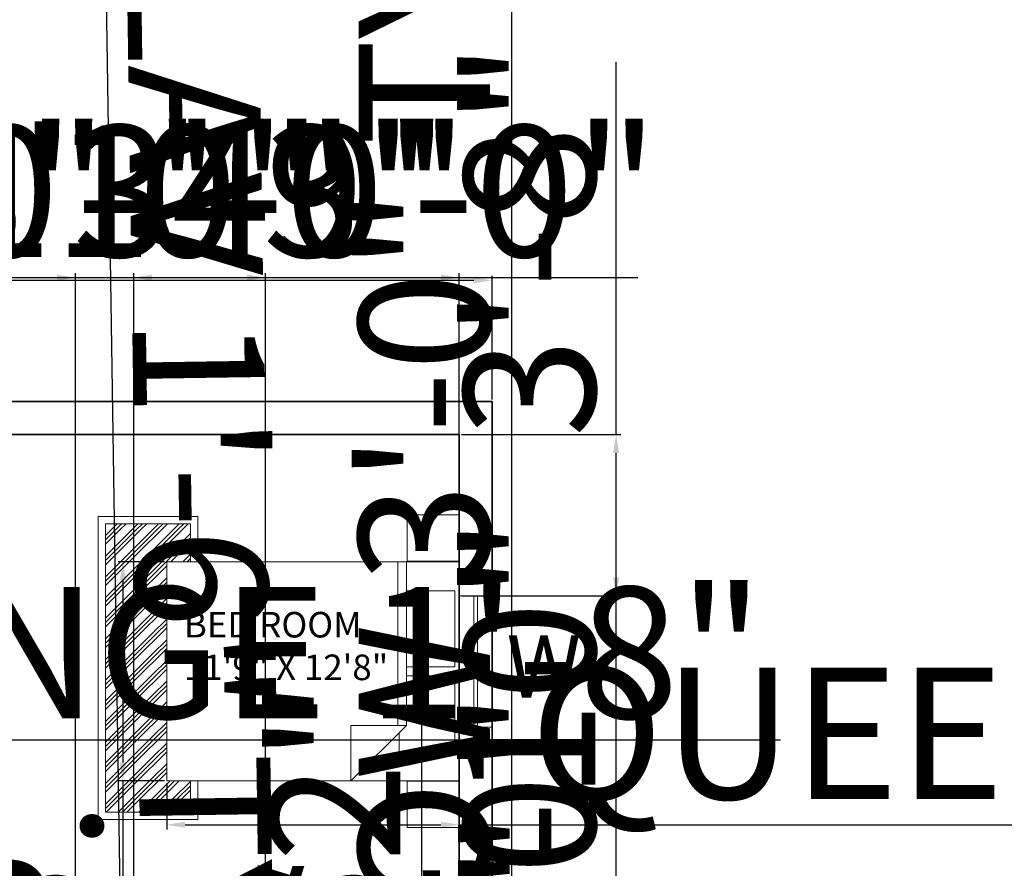
# Model space of a CAD drawing. Units: inches. Extents: x 2901 to 21549, y 2042 to 3828.
# Tile 8 of 10: x 3505 to 3774, y 3347 to 3579. Entities that reach past the tile are written whole.
import ezdxf

# ---------------------------------------------------------------- set-up
doc = ezdxf.new("R2010")
doc.units = ezdxf.units.IN
doc.layers.get('Defpoints').update_dxf_attribs({"color": 1})
for name, color, linetype, lineweight in [('A-ANNO-DIMS', 2, 'Continuous', 18), ('A-ANNO-TEXT', 7, 'Continuous', 18), ('A-AREA-IDEN', 7, 'Continuous', 18), ('A-FLOR-PATT', 252, 'Continuous', 13), ('A-FURN', 8, 'Continuous', 18), ('A-GLAZ', 4, 'Continuous', 18), ('A-WALL', 7, 'Continuous', 35)]:
    doc.layers.add(name, color=color, linetype=linetype, lineweight=lineweight)
doc.styles.get("Standard").update_dxf_attribs({"font": 'arial.ttf'})
doc.dimstyles.new('ISO-25', dxfattribs={"dimtxt": 36, "dimasz": 5, "dimexe": 1.25, "dimexo": 0.625, "dimtad": 1, "dimdec": 0, "dimlunit": 3, "dimtxsty": 'Standard', "dimcen": 2.5, "dimadec": 0, "dimazin": 0, "dimtfac": 1, "dimtdec": 0, "dimtmove": 0, "dimatfit": 3, "dimfxl": 1, "dimarcsym": 0})

# ---------------------------------------------------------------- blocks, each defined once
blk = doc.blocks.new('Bed - Queen')
for p, q in [((0, -80.00003), (0, 0)), ((0, 0), (59.99999, 0)), ((59.99999, 0), (59.99999, -80.00003)), ((7.99999, -1.2), (28.79998, -1.2)), ((7.99999, -14.4), (7.99999, -1.2)), ((28.79998, -1.2), (28.79998, -14.4)), ((31.19999, -1.2), (51.99999, -1.2)), ((31.19999, -14.4), (31.19999, -1.2)), ((51.99999, -1.2), (51.99999, -16.4)), ((0, -14.4), (44.8, -14.4)), ((59.99999, -29.6), (44.8, -14.4)), ((44.8, -14.4), (44.8, -29.6)), ((44.8, -16.8), (0, -16.8)), ((51.99999, -16.4), (46.79936, -16.4)), ((44.8, -29.6), (59.99999, -29.6)), ((59.99999, -80.00003), (0, -80.00003))]:
    blk.add_line(p, q)
blk = doc.blocks.new('*D30')
at = {"layer": 'A-ANNO-DIMS', "color": 0, "lineweight": -2, "transparency": 16777216}
for p, q in [((3334.07, 3475.1), (3334.07, 3508.95)), ((3339.07, 3507.7), (3629.07, 3507.7)), ((3634.07, 3475.1), (3634.07, 3508.95))]:
    blk.add_line(p, q, dxfattribs=at)
at = {"layer": 'A-ANNO-DIMS', "color": 0, "transparency": 16777216}
for points in [[(3339.07, 3508.53), (3339.07, 3506.87), (3334.07, 3507.7)], [(3629.07, 3508.53), (3629.07, 3506.87), (3634.07, 3507.7)]]:
    blk.add_solid(points, dxfattribs=at)
at = {"layer": 'Defpoints', "color": 0, "transparency": 16777216}
for p in [(3634.07, 3507.7), (3334.07, 3474.48), (3634.07, 3474.48)]:
    blk.add_point(p, dxfattribs=at)
at = {"layer": 'A-ANNO-DIMS', "color": 0, "transparency": 16777216, "insert": (3484.07, 3526.7), "char_height": 36, "attachment_point": 5}
blk.add_mtext("25'", dxfattribs=at)
blk = doc.blocks.new('WIN-36IN-9IN-WALL')
for p, q in [((0, 36), (9, 36)), ((0, 0), (0, 36)), ((4, 0), (4, 36)), ((5, 36), (5, 0)), ((9, 36), (9, 0)), ((9, 0), (0, 0))]:
    blk.add_line(p, q)
blk = doc.blocks.new('TABLE-BEDSIDE')
blk.add_lwpolyline([(0, 12.7), (14.22, 12.7), (14.22, 0), (0, 0)], close=True)
blk = doc.blocks.new('*D36')
at = {"layer": 'A-ANNO-DIMS', "color": 0, "lineweight": -2, "transparency": 16777216}
for p, q in [((3639.47, 3192.64), (3639.47, 3654.44)), ((3634.69, 3192.64), (3640.72, 3192.64)), ((3639.47, 3161.64), (3639.47, 3187.64)), ((3634.69, 3156.64), (3640.72, 3156.64))]:
    blk.add_line(p, q, dxfattribs=at)
at = {"layer": 'A-ANNO-DIMS', "color": 0, "transparency": 16777216}
for points in [[(3638.64, 3187.64), (3640.3, 3187.64), (3639.47, 3192.64)], [(3638.64, 3161.64), (3640.3, 3161.64), (3639.47, 3156.64)]]:
    blk.add_solid(points, dxfattribs=at)
at = {"layer": 'Defpoints', "color": 0, "transparency": 16777216}
for p in [(3634.07, 3192.64), (3639.47, 3192.64), (3634.07, 3156.64)]:
    blk.add_point(p, dxfattribs=at)
at = {"layer": 'A-ANNO-DIMS', "color": 0, "transparency": 16777216, "insert": (3620.21, 3426.04), "char_height": 36, "attachment_point": 5, "rotation": 90}
blk.add_mtext('WINDOW 3\'-0" TYP.', dxfattribs=at)
blk = doc.blocks.new('*D42')
at = {"layer": 'A-ANNO-DIMS', "color": 0, "lineweight": -2, "transparency": 16777216}
for p, q in [((3533.42, 3266.44), (3528.38, 3599.53)), ((3535.49, 3266.47), (3532.17, 3266.42)), ((3533.62, 3253.49), (3533.5, 3261.44)), ((3535.76, 3248.52), (3532.44, 3248.47))]:
    blk.add_line(p, q, dxfattribs=at)
at = {"layer": 'A-ANNO-DIMS', "color": 0, "transparency": 16777216}
for points in [[(3534.33, 3261.45), (3532.66, 3261.43), (3533.42, 3266.44)], [(3534.45, 3253.5), (3532.78, 3253.48), (3533.69, 3248.49)]]:
    blk.add_solid(points, dxfattribs=at)
at = {"layer": 'Defpoints', "color": 0, "transparency": 16777216}
for p in [(3533.42, 3266.44), (3536.11, 3266.48), (3536.39, 3248.53)]:
    blk.add_point(p, dxfattribs=at)
at = {"layer": 'A-ANNO-DIMS', "color": 0, "transparency": 16777216, "insert": (3549.86, 3435.77), "char_height": 36, "attachment_point": 5, "rotation": 270.8679}
blk.add_mtext('LAV 1\'-6" TYP.', dxfattribs=at)
blk = doc.blocks.new('*D43')
at = {"layer": 'A-ANNO-DIMS', "color": 0, "lineweight": -2, "transparency": 16777216}
for p, q in [((3550.8, 3269.4), (3856.95, 3274.04)), ((3536.1, 3267.11), (3536.05, 3270.42)), ((3550.83, 3267.33), (3550.78, 3270.65)), ((3541.07, 3269.25), (3545.8, 3269.32))]:
    blk.add_line(p, q, dxfattribs=at)
at = {"layer": 'A-ANNO-DIMS', "color": 0, "transparency": 16777216}
for points in [[(3541.06, 3270.08), (3541.09, 3268.42), (3536.07, 3269.17)], [(3545.78, 3270.16), (3545.81, 3268.49), (3550.8, 3269.4)]]:
    blk.add_solid(points, dxfattribs=at)
at = {"layer": 'Defpoints', "color": 0, "transparency": 16777216}
for p in [(3550.8, 3269.4), (3536.11, 3266.48), (3550.84, 3266.71)]:
    blk.add_point(p, dxfattribs=at)
at = {"layer": 'A-ANNO-DIMS', "color": 0, "transparency": 16777216, "insert": (3706.08, 3290.99), "char_height": 36, "attachment_point": 5, "rotation": 0.8679}
blk.add_mtext('1\'-2 1/2" TYP.', dxfattribs=at)
blk = doc.blocks.new('*D45')
at = {"layer": 'A-ANNO-DIMS', "color": 0, "lineweight": -2, "transparency": 16777216}
for p, q in [((3424.19, 3301.6), (3424.19, 3303.72)), ((3430.69, 3301.6), (3430.69, 3303.72)), ((3419.19, 3302.47), (3414.19, 3302.47)), ((3424.19, 3302.47), (3430.69, 3302.47)), ((3435.69, 3302.47), (3745.26, 3302.47))]:
    blk.add_line(p, q, dxfattribs=at)
at = {"layer": 'A-ANNO-DIMS', "color": 0, "transparency": 16777216}
for points in [[(3419.19, 3303.31), (3419.19, 3301.64), (3424.19, 3302.47)], [(3435.69, 3303.31), (3435.69, 3301.64), (3430.69, 3302.47)]]:
    blk.add_solid(points, dxfattribs=at)
at = {"layer": 'Defpoints', "color": 0, "transparency": 16777216}
for p in [(3424.19, 3300.97), (3430.69, 3302.47), (3430.69, 3300.97)]:
    blk.add_point(p, dxfattribs=at)
at = {"layer": 'A-ANNO-DIMS', "color": 0, "transparency": 16777216, "insert": (3592.98, 3321.71), "char_height": 36, "attachment_point": 5}
blk.add_mtext('0\'-6 1/2" TYP.', dxfattribs=at)
blk = doc.blocks.new('*D46')
at = {"layer": 'A-ANNO-DIMS', "color": 0, "lineweight": -2, "transparency": 16777216}
for p, q in [((3545.07, 3370.05), (3545.07, 3357.42)), ((3625.07, 3370.05), (3625.07, 3357.42)), ((3550.07, 3358.67), (3620.07, 3358.67)), ((3625.07, 3358.67), (4160.88, 3358.67))]:
    blk.add_line(p, q, dxfattribs=at)
at = {"layer": 'A-ANNO-DIMS', "color": 0, "transparency": 16777216}
for points in [[(3550.07, 3359.51), (3550.07, 3357.84), (3545.07, 3358.67)], [(3620.07, 3359.51), (3620.07, 3357.84), (3625.07, 3358.67)]]:
    blk.add_solid(points, dxfattribs=at)
at = {"layer": 'Defpoints', "color": 0, "transparency": 16777216}
for p in [(3545.07, 3370.67), (3625.07, 3370.67), (3625.07, 3358.67)]:
    blk.add_point(p, dxfattribs=at)
at = {"layer": 'A-ANNO-DIMS', "color": 0, "transparency": 16777216, "insert": (3895.48, 3379.02), "char_height": 36, "attachment_point": 5}
blk.add_mtext('QUEEN BED 6\'-8" TYP.', dxfattribs=at)
blk = doc.blocks.new('*D47')
at = {"layer": 'A-ANNO-DIMS', "color": 0, "lineweight": -2, "transparency": 16777216}
for p, q in [((3544.44, 3430.67), (3531.82, 3430.67)), ((3533.07, 3425.67), (3533.07, 3375.67)), ((3544.44, 3370.67), (3531.82, 3370.67)), ((3533.07, 3370.67), (3533.07, 3144.99))]:
    blk.add_line(p, q, dxfattribs=at)
at = {"layer": 'A-ANNO-DIMS', "color": 0, "transparency": 16777216}
for points in [[(3532.24, 3425.67), (3533.9, 3425.67), (3533.07, 3430.67)], [(3532.24, 3375.67), (3533.9, 3375.67), (3533.07, 3370.67)]]:
    blk.add_solid(points, dxfattribs=at)
at = {"layer": 'Defpoints', "color": 0, "transparency": 16777216}
for p in [(3545.07, 3430.67), (3533.07, 3370.67), (3545.07, 3370.67)]:
    blk.add_point(p, dxfattribs=at)
at = {"layer": 'A-ANNO-DIMS', "color": 0, "transparency": 16777216, "insert": (3514.06, 3255.33), "char_height": 36, "attachment_point": 5, "rotation": 90}
blk.add_mtext('5\'-0" TYP.', dxfattribs=at)
blk = doc.blocks.new('*D55')
at = {"layer": 'A-ANNO-DIMS', "color": 0, "lineweight": -2, "transparency": 16777216}
for p, q in [((3614.88, 3206.89), (3614.88, 3392.69)), ((3605.24, 3206.89), (3616.13, 3206.89)), ((3614.88, 3170.49), (3614.88, 3201.89)), ((3605.24, 3165.49), (3616.13, 3165.49))]:
    blk.add_line(p, q, dxfattribs=at)
at = {"layer": 'A-ANNO-DIMS', "color": 0, "transparency": 16777216}
for points in [[(3614.05, 3201.89), (3615.72, 3201.89), (3614.88, 3206.89)], [(3614.05, 3170.49), (3615.72, 3170.49), (3614.88, 3165.49)]]:
    blk.add_solid(points, dxfattribs=at)
at = {"layer": 'Defpoints', "color": 0, "transparency": 16777216}
for p in [(3604.61, 3206.89), (3614.88, 3206.89), (3604.61, 3165.49)]:
    blk.add_point(p, dxfattribs=at)
at = {"layer": 'A-ANNO-DIMS', "color": 0, "transparency": 16777216, "insert": (3595.63, 3302.29), "char_height": 36, "attachment_point": 5, "rotation": 90}
blk.add_mtext('3\'-5 1/2"', dxfattribs=at)
blk = doc.blocks.new('*D58')
at = {"layer": 'A-ANNO-DIMS', "color": 0, "lineweight": -2, "transparency": 16777216}
for p, q in [((3399.98, 3384.28), (3399.98, 3380.64)), ((3420.08, 3384.28), (3420.08, 3380.64)), ((3404.98, 3381.89), (3415.08, 3381.89)), ((3420.08, 3381.89), (3712.98, 3381.89))]:
    blk.add_line(p, q, dxfattribs=at)
at = {"layer": 'A-ANNO-DIMS', "color": 0, "transparency": 16777216}
for points in [[(3404.98, 3382.72), (3404.98, 3381.06), (3399.98, 3381.89)], [(3415.08, 3382.72), (3415.08, 3381.06), (3420.08, 3381.89)]]:
    blk.add_solid(points, dxfattribs=at)
at = {"layer": 'Defpoints', "color": 0, "transparency": 16777216}
for p in [(3399.98, 3384.91), (3420.08, 3384.91), (3420.08, 3381.89)]:
    blk.add_point(p, dxfattribs=at)
at = {"layer": 'A-ANNO-DIMS', "color": 0, "transparency": 16777216, "insert": (3569.03, 3401.13), "char_height": 36, "attachment_point": 5}
blk.add_mtext('RANGE 1\'-8"', dxfattribs=at)
blk = doc.blocks.new('*D67')
at = {"layer": 'A-ANNO-DIMS', "color": 0, "lineweight": -2, "transparency": 16777216}
for p, q in [((3484.07, 3013.1), (3484.07, 3509.68)), ((3489.07, 3508.43), (3620.07, 3508.43)), ((3625.07, 3228.1), (3625.07, 3509.68))]:
    blk.add_line(p, q, dxfattribs=at)
at = {"layer": 'A-ANNO-DIMS', "color": 0, "transparency": 16777216}
for points in [[(3489.07, 3509.26), (3489.07, 3507.59), (3484.07, 3508.43)], [(3620.07, 3509.26), (3620.07, 3507.59), (3625.07, 3508.43)]]:
    blk.add_solid(points, dxfattribs=at)
at = {"layer": 'Defpoints', "color": 0, "transparency": 16777216}
for p in [(3625.07, 3508.43), (3625.07, 3227.48), (3484.07, 3012.48)]:
    blk.add_point(p, dxfattribs=at)
at = {"layer": 'A-ANNO-DIMS', "color": 0, "transparency": 16777216, "insert": (3554.57, 3527.43), "char_height": 36, "attachment_point": 5}
blk.add_mtext('11\'-9"', dxfattribs=at)
blk = doc.blocks.new('*D69')
at = {"layer": 'A-ANNO-DIMS', "color": 0, "lineweight": -2, "transparency": 16777216}
for p, q in [((3668.02, 3287.47), (3668.02, 3390.03)), ((3634.69, 3287.47), (3669.27, 3287.47)), ((3668.02, 3268.47), (3668.02, 3282.47)), ((3634.69, 3263.47), (3669.27, 3263.47))]:
    blk.add_line(p, q, dxfattribs=at)
at = {"layer": 'A-ANNO-DIMS', "color": 0, "transparency": 16777216}
for points in [[(3667.19, 3282.47), (3668.85, 3282.47), (3668.02, 3287.47)], [(3667.19, 3268.47), (3668.85, 3268.47), (3668.02, 3263.47)]]:
    blk.add_solid(points, dxfattribs=at)
at = {"layer": 'Defpoints', "color": 0, "transparency": 16777216}
for p in [(3634.07, 3287.47), (3668.02, 3287.47), (3634.07, 3263.47)]:
    blk.add_point(p, dxfattribs=at)
at = {"layer": 'A-ANNO-DIMS', "color": 0, "transparency": 16777216, "insert": (3649.01, 3341.25), "char_height": 36, "attachment_point": 5, "rotation": 90}
blk.add_mtext('2\'-0"', dxfattribs=at)
blk = doc.blocks.new('*D70')
at = {"layer": 'A-ANNO-DIMS', "color": 0, "lineweight": -2, "transparency": 16777216}
for p, q in [((3668.02, 3309.48), (3668.02, 3436.01)), ((3625.69, 3309.48), (3669.27, 3309.48)), ((3668.02, 3292.47), (3668.02, 3304.48)), ((3625.69, 3287.47), (3669.27, 3287.47))]:
    blk.add_line(p, q, dxfattribs=at)
at = {"layer": 'A-ANNO-DIMS', "color": 0, "transparency": 16777216}
for points in [[(3667.19, 3304.48), (3668.85, 3304.48), (3668.02, 3309.48)], [(3667.19, 3292.47), (3668.85, 3292.47), (3668.02, 3287.47)]]:
    blk.add_solid(points, dxfattribs=at)
at = {"layer": 'Defpoints', "color": 0, "transparency": 16777216}
for p in [(3625.07, 3309.48), (3668.02, 3309.48), (3625.07, 3287.47)]:
    blk.add_point(p, dxfattribs=at)
at = {"layer": 'A-ANNO-DIMS', "color": 0, "transparency": 16777216, "insert": (3649.01, 3375.24), "char_height": 36, "attachment_point": 5, "rotation": 90}
blk.add_mtext('1\'-10"', dxfattribs=at)
blk = doc.blocks.new('*D71')
at = {"layer": 'A-ANNO-DIMS', "color": 0, "lineweight": -2, "transparency": 16777216}
for p, q in [((3536.07, 3310.1), (3536.07, 3509.68)), ((3541.07, 3508.43), (3567.07, 3508.43)), ((3572.07, 3310.1), (3572.07, 3509.68)), ((3572.07, 3508.43), (3673.99, 3508.43))]:
    blk.add_line(p, q, dxfattribs=at)
at = {"layer": 'A-ANNO-DIMS', "color": 0, "transparency": 16777216}
for points in [[(3541.07, 3509.26), (3541.07, 3507.59), (3536.07, 3508.43)], [(3567.07, 3509.26), (3567.07, 3507.59), (3572.07, 3508.43)]]:
    blk.add_solid(points, dxfattribs=at)
at = {"layer": 'Defpoints', "color": 0, "transparency": 16777216}
for p in [(3572.07, 3508.43), (3536.07, 3309.48), (3572.07, 3309.48)]:
    blk.add_point(p, dxfattribs=at)
at = {"layer": 'A-ANNO-DIMS', "color": 0, "transparency": 16777216, "insert": (3625.53, 3527.45), "char_height": 36, "attachment_point": 5}
blk.add_mtext('3\'-0"', dxfattribs=at)
blk = doc.blocks.new('*D72')
at = {"layer": 'A-ANNO-DIMS', "color": 0, "lineweight": -2, "transparency": 16777216}
for p, q in [((3668.02, 3465.48), (3668.02, 3567.4)), ((3625.69, 3465.48), (3669.27, 3465.48)), ((3668.02, 3426.34), (3668.02, 3460.48)), ((3625.69, 3421.34), (3669.27, 3421.34))]:
    blk.add_line(p, q, dxfattribs=at)
at = {"layer": 'A-ANNO-DIMS', "color": 0, "transparency": 16777216}
for points in [[(3667.19, 3460.48), (3668.85, 3460.48), (3668.02, 3465.48)], [(3667.19, 3426.34), (3668.85, 3426.34), (3668.02, 3421.34)]]:
    blk.add_solid(points, dxfattribs=at)
at = {"layer": 'Defpoints', "color": 0, "transparency": 16777216}
for p in [(3625.07, 3465.48), (3668.02, 3465.48), (3625.07, 3421.34)]:
    blk.add_point(p, dxfattribs=at)
at = {"layer": 'A-ANNO-DIMS', "color": 0, "transparency": 16777216, "insert": (3649, 3518.94), "char_height": 36, "attachment_point": 5, "rotation": 90}
blk.add_mtext('3\'-8"', dxfattribs=at)
blk = doc.blocks.new('*D74')
at = {"layer": 'A-ANNO-DIMS', "color": 0, "lineweight": -2, "transparency": 16777216}
for p, q in [((3668.02, 3227.48), (3668.02, 3358.01)), ((3625.69, 3227.48), (3669.27, 3227.48)), ((3668.02, 3197.64), (3668.02, 3222.48)), ((3625.69, 3192.64), (3669.27, 3192.64))]:
    blk.add_line(p, q, dxfattribs=at)
at = {"layer": 'A-ANNO-DIMS', "color": 0, "transparency": 16777216}
for points in [[(3667.19, 3222.48), (3668.85, 3222.48), (3668.02, 3227.48)], [(3667.19, 3197.64), (3668.85, 3197.64), (3668.02, 3192.64)]]:
    blk.add_solid(points, dxfattribs=at)
at = {"layer": 'Defpoints', "color": 0, "transparency": 16777216}
for p in [(3625.07, 3227.48), (3668.02, 3227.48), (3625.07, 3192.64)]:
    blk.add_point(p, dxfattribs=at)
at = {"layer": 'A-ANNO-DIMS', "color": 0, "transparency": 16777216, "insert": (3649.32, 3295.24), "char_height": 36, "attachment_point": 5, "rotation": 90}
blk.add_mtext('2\'-11"', dxfattribs=at)
blk = doc.blocks.new('*D77')
at = {"layer": 'A-ANNO-DIMS', "color": 0, "lineweight": -2, "transparency": 16777216}
for p, q in [((3475.07, 3508.43), (3470.07, 3508.43)), ((3480.07, 3310.1), (3480.07, 3509.68)), ((3480.07, 3508.43), (3484.07, 3508.43)), ((3484.07, 3310.1), (3484.07, 3509.68)), ((3489.07, 3508.43), (3591.02, 3508.43))]:
    blk.add_line(p, q, dxfattribs=at)
at = {"layer": 'A-ANNO-DIMS', "color": 0, "transparency": 16777216}
for points in [[(3475.07, 3509.26), (3475.07, 3507.59), (3480.07, 3508.43)], [(3489.07, 3509.26), (3489.07, 3507.59), (3484.07, 3508.43)]]:
    blk.add_solid(points, dxfattribs=at)
at = {"layer": 'Defpoints', "color": 0, "transparency": 16777216}
for p in [(3484.07, 3508.43), (3480.07, 3309.48), (3484.07, 3309.48)]:
    blk.add_point(p, dxfattribs=at)
at = {"layer": 'A-ANNO-DIMS', "color": 0, "transparency": 16777216, "insert": (3542.54, 3527.43), "char_height": 36, "attachment_point": 5}
blk.add_mtext('0\'-4"', dxfattribs=at)
blk = doc.blocks.new('*D81')
at = {"layer": 'A-ANNO-DIMS', "color": 0, "lineweight": -2, "transparency": 16777216}
for p, q in [((3444.07, 3314.1), (3444.07, 3509.68)), ((3449.07, 3508.43), (3475.07, 3508.43)), ((3480.07, 3314.1), (3480.07, 3509.68)), ((3480.07, 3508.43), (3581.99, 3508.43))]:
    blk.add_line(p, q, dxfattribs=at)
at = {"layer": 'A-ANNO-DIMS', "color": 0, "transparency": 16777216}
for points in [[(3449.07, 3509.26), (3449.07, 3507.59), (3444.07, 3508.43)], [(3475.07, 3509.26), (3475.07, 3507.59), (3480.07, 3508.43)]]:
    blk.add_solid(points, dxfattribs=at)
at = {"layer": 'Defpoints', "color": 0, "transparency": 16777216}
for p in [(3480.07, 3508.43), (3444.07, 3313.48), (3480.07, 3313.48)]:
    blk.add_point(p, dxfattribs=at)
at = {"layer": 'A-ANNO-DIMS', "color": 0, "transparency": 16777216, "insert": (3533.53, 3527.45), "char_height": 36, "attachment_point": 5}
blk.add_mtext('3\'-0"', dxfattribs=at)
blk = doc.blocks.new('*D82')
at = {"layer": 'A-ANNO-DIMS', "color": 0, "lineweight": -2, "transparency": 16777216}
for p, q in [((3484.07, 3313.93), (3484.07, 3509.68)), ((3489.07, 3508.43), (3515.07, 3508.43)), ((3520.07, 3314.1), (3520.07, 3509.68)), ((3520.07, 3508.43), (3621.99, 3508.43))]:
    blk.add_line(p, q, dxfattribs=at)
at = {"layer": 'A-ANNO-DIMS', "color": 0, "transparency": 16777216}
for points in [[(3489.07, 3509.26), (3489.07, 3507.59), (3484.07, 3508.43)], [(3515.07, 3509.26), (3515.07, 3507.59), (3520.07, 3508.43)]]:
    blk.add_solid(points, dxfattribs=at)
at = {"layer": 'Defpoints', "color": 0, "transparency": 16777216}
for p in [(3520.07, 3508.43), (3484.07, 3313.3), (3520.07, 3313.48)]:
    blk.add_point(p, dxfattribs=at)
at = {"layer": 'A-ANNO-DIMS', "color": 0, "transparency": 16777216, "insert": (3573.53, 3527.45), "char_height": 36, "attachment_point": 5}
blk.add_mtext('3\'-0"', dxfattribs=at)

msp = doc.modelspace()

# ---------------------------------------------------------------- hatches: boundary and pattern name
at = {"layer": 'A-FLOR-PATT'}
h = msp.add_hatch(dxfattribs=at)
h.set_pattern_fill('GOST_GROUND', color=256, scale=0.4)
h.paths.add_polyline_path([(3545.07, 3430.67), (3551.56, 3430.67), (3551.56, 3441.03), (3528.35, 3441.03), (3528.35, 3362.09), (3551.56, 3362.09), (3551.56, 3370.67), (3545.07, 3370.67)])

# ---------------------------------------------------------------- linework, layer by layer
at = {"layer": 'A-FURN'}
for points in [[(3553.56, 3370.67), (3553.56, 3360.09), (3526.35, 3360.09), (3526.35, 3443.03), (3553.56, 3443.03), (3553.56, 3430.67)], [(3551.56, 3370.67), (3551.56, 3362.09), (3528.35, 3362.09), (3528.35, 3441.03), (3551.56, 3441.03), (3551.56, 3430.67)]]:
    msp.add_lwpolyline(points, dxfattribs=at)
at = {"layer": 'A-WALL'}
for p, q in [((3343.07, 3465.48), (3625.07, 3465.48)), ((3625.07, 3465.48), (3625.07, 2883.48))]:
    msp.add_line(p, q, dxfattribs=at)
msp.add_lwpolyline([(3634.07, 3474.48), (3634.07, 2874.48), (3334.07, 2874.48), (3334.07, 3474.48)], close=True, dxfattribs=at)

# ---------------------------------------------------------------- block references
at = {"layer": 'A-FURN'}
for p in [(3610.83, 3430.8), (3610.83, 3357.93)]:
    msp.add_blockref('TABLE-BEDSIDE', p, dxfattribs=at)
at = {"layer": 'A-FURN', "rotation": 270}
msp.add_blockref('Bed - Queen', (3625.07, 3430.67), dxfattribs=at)
at = {"layer": 'A-GLAZ'}
msp.add_blockref('WIN-36IN-9IN-WALL', (3625.07, 3385.34), dxfattribs=at)

# ---------------------------------------------------------------- texts
at = {"layer": 'A-ANNO-TEXT', "insert": (3638.04, 3410.49), "char_height": 17, "attachment_point": 1}
msp.add_mtext_dynamic_manual_height_columns('{\\fArial|b1|i0|c0|p34;W}', width=86.7973, gutter_width=12.5, heights=[27.4], dxfattribs=at)
at = {"layer": 'A-AREA-IDEN', "insert": (3549.77, 3416.93), "char_height": 7, "attachment_point": 1}
msp.add_mtext_dynamic_manual_height_columns('{\\fArial|b1|i0|c0|p34;BED ROOM\\P11\'9" X 12\'8"}', width=86.7973, gutter_width=12.5, heights=[27.4], dxfattribs=at)

# ---------------------------------------------------------------- dimensions: what is measured, and where the dimension line sits
at = {"layer": 'A-ANNO-DIMS'}
for base, p1, p2, angle, text, picture, middle in [((3639.47, 3192.64), (3634.07, 3156.64), (3634.07, 3192.64), 90, 'WINDOW <> TYP.', '*D36', (3620.21, 3426.04)), ((3533.42, 3266.44), (3536.39, 3248.53), (3536.11, 3266.48), 90.8679, 'LAV <> TYP.', '*D42', (3549.86, 3435.77)), ((3533.07, 3370.67), (3545.07, 3430.67), (3545.07, 3370.67), 270, '<> TYP.', '*D47', (3514.06, 3255.33)), ((3550.8, 3269.4), (3536.11, 3266.48), (3550.84, 3266.71), 0.8679, '<> TYP.', '*D43', (3706.08, 3290.99))]:
    dim = msp.add_linear_dim(base=base, p1=p1, p2=p2, angle=angle, text=text, dimstyle='ISO-25', override={"dimdec": 1, "dimlfac": 1, "dimrnd": 0, "dimzin": 1, "dimdsep": 46, "dimlunit": 4, "dimfrac": 2}, dxfattribs=at)
    dim.commit()
    dim.dimension.update_dxf_attribs({"geometry": picture, "text_midpoint": middle})
for base, p1, p2, picture, middle in [((3668.02, 3465.48), (3625.07, 3421.34), (3625.07, 3465.48), '*D72', (3649, 3518.94)), ((3668.02, 3309.48), (3625.07, 3287.47), (3625.07, 3309.48), '*D70', (3649.01, 3375.24)), ((3614.88, 3206.89), (3604.61, 3165.49), (3604.61, 3206.89), '*D55', (3595.63, 3302.29)), ((3668.02, 3287.47), (3634.07, 3263.47), (3634.07, 3287.47), '*D69', (3649.01, 3341.25)), ((3668.02, 3227.48), (3625.07, 3192.64), (3625.07, 3227.48), '*D74', (3649.32, 3295.24))]:
    dim = msp.add_linear_dim(base=base, p1=p1, p2=p2, angle=90, dimstyle='ISO-25', override={"dimdec": 1, "dimlfac": 1, "dimrnd": 0, "dimzin": 1, "dimdsep": 46, "dimlunit": 4, "dimfrac": 2}, dxfattribs=at)
    dim.commit()
    dim.dimension.update_dxf_attribs({"geometry": picture, "text_midpoint": middle})
for base, p1, p2, override, picture, middle in [((3634.07, 3507.7), (3334.07, 3474.48), (3634.07, 3474.48), {"dimclrd": 0, "dimclre": 0, "dimclrt": 0}, '*D30', (3484.07, 3526.7)), ((3480.07, 3508.43), (3444.07, 3313.48), (3480.07, 3313.48), {"dimdec": 1, "dimlfac": 1, "dimrnd": 0, "dimzin": 1, "dimdsep": 46, "dimlunit": 4, "dimfrac": 2}, '*D81', (3533.53, 3527.45)), ((3484.07, 3508.43), (3480.07, 3309.48), (3484.07, 3309.48), {"dimdec": 1, "dimlfac": 1, "dimrnd": 0, "dimzin": 1, "dimdsep": 46, "dimlunit": 4, "dimfrac": 2}, '*D77', (3542.54, 3527.43)), ((3520.07, 3508.43), (3484.07, 3313.3), (3520.07, 3313.48), {"dimdec": 1, "dimlfac": 1, "dimrnd": 0, "dimzin": 1, "dimdsep": 46, "dimlunit": 4, "dimfrac": 2}, '*D82', (3573.53, 3527.45)), ((3625.07, 3508.43), (3484.07, 3012.48), (3625.07, 3227.48), {"dimdec": 1, "dimlfac": 1, "dimrnd": 0, "dimzin": 1, "dimdsep": 46, "dimlunit": 4, "dimfrac": 2}, '*D67', (3554.57, 3527.43)), ((3572.07, 3508.43), (3536.07, 3309.48), (3572.07, 3309.48), {"dimdec": 1, "dimlfac": 1, "dimrnd": 0, "dimzin": 1, "dimdsep": 46, "dimlunit": 4, "dimfrac": 2}, '*D71', (3625.53, 3527.45))]:
    dim = msp.add_linear_dim(base=base, p1=p1, p2=p2, dimstyle='ISO-25', override=override, dxfattribs=at)
    dim.commit()
    dim.dimension.update_dxf_attribs({"geometry": picture, "text_midpoint": middle})
for base, p1, p2, text, picture, middle in [((3625.07, 3358.67), (3545.07, 3370.67), (3625.07, 3370.67), 'QUEEN BED <> TYP.', '*D46', (3895.48, 3379.02)), ((3420.08, 3381.89), (3399.98, 3384.91), (3420.08, 3384.91), 'RANGE <>', '*D58', (3569.03, 3401.13)), ((3430.69, 3302.47), (3424.19, 3300.97), (3430.69, 3300.97), '<> TYP.', '*D45', (3592.98, 3321.71))]:
    dim = msp.add_linear_dim(base=base, p1=p1, p2=p2, text=text, dimstyle='ISO-25', override={"dimdec": 1, "dimlfac": 1, "dimrnd": 0, "dimzin": 1, "dimdsep": 46, "dimlunit": 4, "dimfrac": 2}, dxfattribs=at)
    dim.commit()
    dim.dimension.update_dxf_attribs({"geometry": picture, "text_midpoint": middle})

doc.saveas('drawing.dxf')
